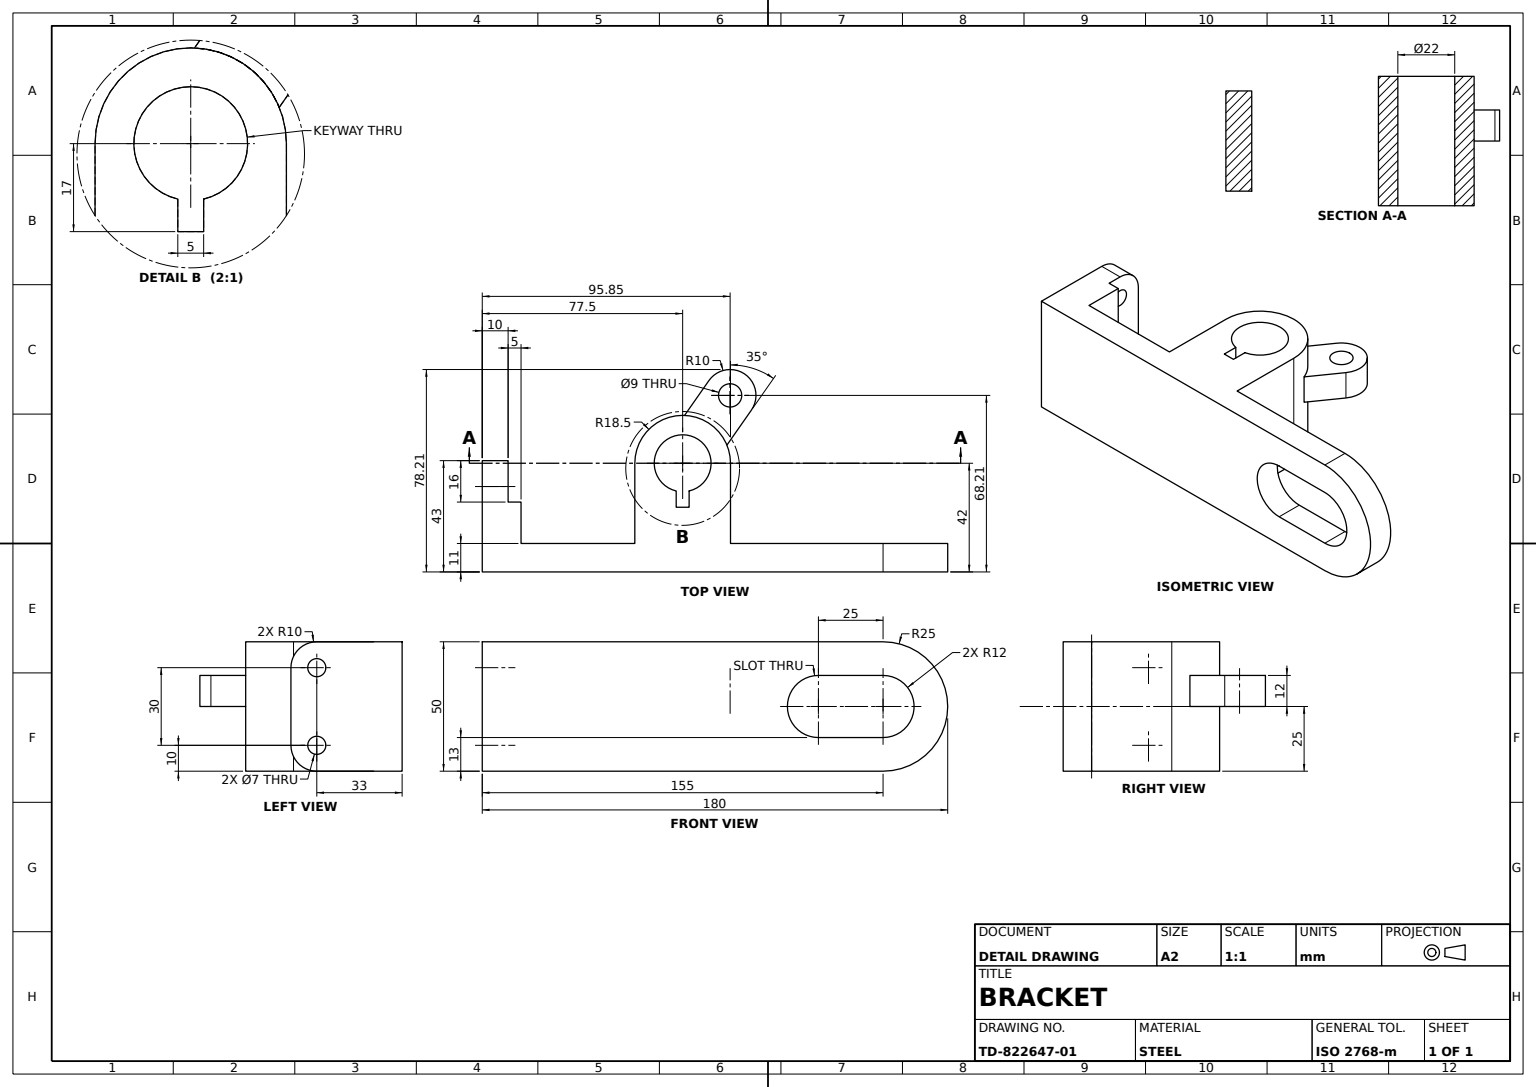
SolidWorks part; units mm, degrees
material "Plain Carbon Steel"
ref_plane "Front Plane" through (0, 0, 0) normal (0, 0, 1) x (1, 0, 0)
ref_plane "Top Plane" through (0, 0, 0) normal (0, 1, 0) x (1, 0, 0)
ref_plane "Right Plane" through (0, 0, 0) normal (1, 0, 0) x (0, 0, -1)
sketch "Slotted Arm Sketch" plane through (0, 0, 0) normal (0, 0, 1) x (1, 0, 0)
  line L0 (-77.5, 0) -> (77.5, 0) construction
  line L1 (-77.5, 25) -> (77.5, 25)
  line L2 (-77.5, -25) -> (77.5, -25)
  line L3 (52.5, 0) -> (77.5, 0) construction
  line L4 (52.5, 12) -> (77.5, 12)
  line L5 (52.5, -12) -> (77.5, -12)
  line L6 (-77.5, 25) -> (-77.5, -25)
  arc A1 (77.5, -25) -> (77.5, 25) centre (77.5, 0) ccw
  arc A2 (52.5, 12) -> (52.5, -12) centre (52.5, 0) ccw
  arc A3 (77.5, -12) -> (77.5, 12) centre (77.5, 0) ccw
  point P2 (0, 0)
  point P10 (65, 0)
  dimension "D2" = 25
  dimension "D1" = 155
  dimension "D3" = 25
  dimension "D4" = 13
extrude "Slotted Arm Plate" add sketch "Slotted Arm Sketch" along normal blind 11
sketch "End Wall Sketch" plane through (0, 0, 0) normal (0, 1, 0) x (1, 0, 0)
  line L0 (-77.5, 0) -> (-77.5, 32)
  line L1 (-77.5, 32) -> (-67.5, 32)
  line L2 (-67.5, 32) -> (-67.5, 16)
  line L3 (-67.5, 16) -> (-62.5, 16)
  line L4 (-62.5, 16) -> (-62.5, 0)
  line L5 (77.5, 0) -> (-77.5, 0) construction
  line L6 (-62.5, 0) -> (-77.5, 0)
  line L7 (77.5, -11) -> (-77.5, -11) construction
  dimension "D1" = 16
  dimension "D2" = 43
  dimension "D3" = 5
  dimension "D4" = 10
extrude "End Wall" add sketch "End Wall Sketch" along normal mid plane 50
fillet "End Wall Fillet R10" radius 10 2 edges at (-72.5, -25, -32) (-72.5, 25, -32)
sketch "Wall Notch Sketch" plane through (-77.5, 0, 0) normal (-1, 0, 0) x (0, 0, 1)
  circle A0 centre (-22, 15) radius 3.5
  circle A1 centre (-22, -15) radius 3.5
  dimension "D1" = 7
  dimension "D2" = 7
extrude "Wall Notch Cut" cut sketch "Wall Notch Sketch" against normal mid plane 50
sketch "Hub Sketch" plane through (0, 0, 0) normal (0, 1, 0) x (1, 0, 0)
  line L0 (0, 0) -> (0, 31) construction
  line L1 (77.5, -11) -> (-77.5, -11) construction
  line L2 (-18.5, 0) -> (-18.5, 31)
  line L3 (18.5, 0) -> (18.5, 31)
  line L4 (-18.5, 0) -> (18.5, 0)
  line L5 (-2.5, 14) -> (2.5, 14)
  line L6 (-2.5, 14) -> (-2.5, 20.2879)
  line L8 (2.5, 14) -> (2.5, 20.2879)
  line L9 (-2.5, 14) -> (0.2219, 20.0022) construction
  line L10 (-0.2219, 20.0022) -> (2.5, 14) construction
  line L11 (0, 31) -> (43.4443, 31) construction
  line L12 (-6.3093, 21.9893) -> (18.3544, 57.2129) construction
  line L15 (0.7358, 49.4854) -> (10.1629, 62.9486)
  line L16 (77.5, 0) -> (-62.5, 0) construction
  line L17 (10.6112, 46.1543) -> (18.417, 57.3022) construction
  line L18 (17.1189, 38.0138) -> (26.546, 51.4771)
  arc A1 (18.5, 31) -> (-18.5, 31) centre (0, 31) ccw
  arc A2 (2.5, 20.2879) -> (-2.5, 20.2879) centre (0, 31) ccw
  arc A3 (-0.2219, 20.0022) -> (0.2219, 20.0022) centre (0, 31) ccw
  arc A5 (26.546, 51.4771) -> (10.1629, 62.9486) centre (18.3544, 57.2129) ccw
  circle A6 centre (18.3544, 57.2129) radius 4.5
  point P5 (0, -11)
  point P12 (0, 19.5129)
  point P22 (0, 31)
  dimension "D2" = 18.5
  dimension "D3" = 22
  dimension "D5" = 17
  dimension "D8" = 10
  dimension "D9" = 9
  dimension "D1" = 18.2781
  dimension "D4" = 5
  dimension "D6" = 19.2358
  dimension "D7" = 28.6629
  dimension "D10" = 35.6189
  dimension "D11" = 14
extrude "Hub With Keyed Bore" add sketch "Hub Sketch" along normal mid plane 50 contours L3 A1 L2 L4 A2 L8 L5 L6
sketch "Eye Lug Sketch" plane through (0, 0, 0) normal (0, 1, 0) x (1, 0, 0)
  line L0 (17.1189, 38.0138) -> (26.546, 51.4771) construction
  line L1 (0.7358, 49.4854) -> (10.1629, 62.9486) construction
  line L2 (17.1189, 38.0138) -> (26.546, 51.4771)
  line L3 (0.7358, 49.4854) -> (10.1629, 62.9486)
  arc A0 (18.5, 31) -> (-18.5, 31) centre (0, 31) ccw construction
  circle A1 centre (18.3544, 57.2129) radius 4.5 construction
  arc A2 (26.546, 51.4771) -> (10.1629, 62.9486) centre (18.3544, 57.2129) ccw construction
  arc A3 (17.1189, 38.0138) -> (0.7358, 49.4854) centre (0, 31) ccw
  circle A4 centre (18.3544, 57.2129) radius 4.5
  arc A5 (26.546, 51.4771) -> (10.1629, 62.9486) centre (18.3544, 57.2129) ccw
extrude "Eye Lug" add sketch "Eye Lug Sketch" along normal blind 12
